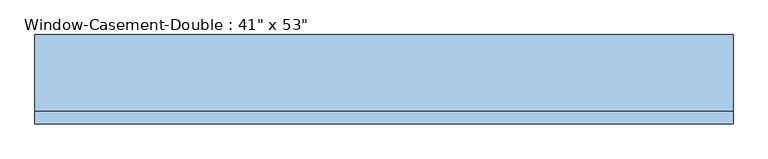
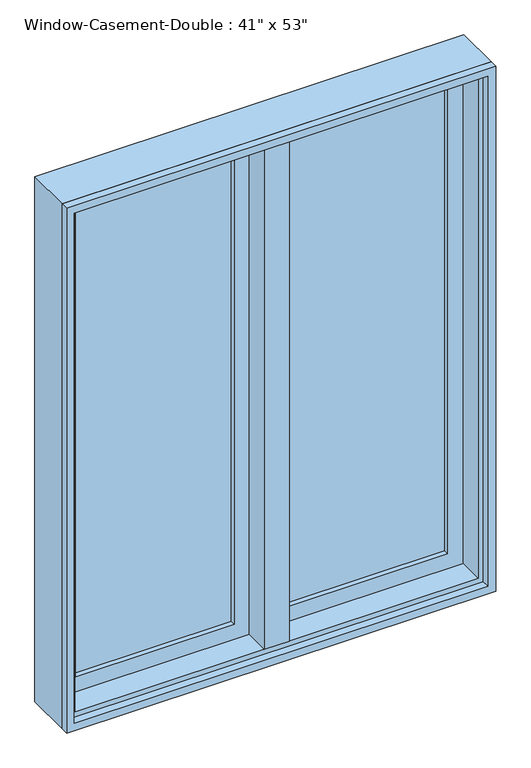
"""IFC4 building model written with IfcOpenShell, lengths in millimetres: window geometry."""

from ifc_helpers import new_model, si_unit, frame, origin, place, context, project, spatial, polyline, outline, extrude, faceted_brep, source, transform, mapped, element, save


def window_8ddb865a(model_context):
    return source(origin(), model_context, "Body", "SolidModel", [
        faceted_brep([(9.525, 76.2, 2247.9), (-9.525, 76.2, 2247.9), (-9.525, 25.4, 2247.9), (9.525, 25.4, 2247.9), (9.525, 76.2, 927.1), (9.525, 25.4, 927.1), (-9.525, 25.4, 927.1), (-9.525, 76.2, 927.1), (-9.525, 25.4, 946.15), (-9.525, 25.4, 2228.85), (-30.1625, 25.4, 946.15), (-30.1625, 25.4, 2228.85), (-30.1625, -38.1, 946.15), (-30.1625, -38.1, 2228.85), (30.1625, -38.1, 946.15), (30.1625, -38.1, 2228.85), (30.1625, 25.4, 946.15), (30.1625, 25.4, 2228.85), (9.525, 25.4, 946.15), (9.525, 25.4, 2228.85)], [[[0, 1, 2, 3]], [[4, 5, 6, 7]], [[1, 0, 4, 7]], [[2, 1, 7, 6, 8, 9]], [[9, 8, 10, 11]], [[11, 10, 12, 13]], [[13, 12, 14, 15]], [[15, 14, 16, 17]], [[17, 16, 18, 19]], [[0, 3, 19, 18, 5, 4]], [[18, 8, 6, 5]], [[9, 19, 3, 2]], [[8, 18, 16, 14, 12, 10]], [[19, 9, 11, 13, 15, 17]]]),
        extrude(outline(polyline([(-66.675, 57.15), (-66.675, 50.8), (-450.85, 50.8), (-450.85, 57.15), (-66.675, 57.15)])), frame((0.0, 0.0, 984.25), z_axis=(0.0, 0.0, 1.0), x_axis=(1.0, 0.0, 0.0)), (0.0, 0.0, 1.0), 1206.5),
        extrude(outline(polyline([(-450.85, 38.1), (-450.85, 44.45), (-66.675, 44.45), (-66.675, 38.1), (-450.85, 38.1)])), frame((0.0, 0.0, 984.25), z_axis=(0.0, 0.0, 1.0), x_axis=(1.0, 0.0, 0.0)), (0.0, 0.0, 1.0), 1206.5),
        extrude(outline(polyline([(450.85, 57.15), (450.85, 50.8), (66.675, 50.8), (66.675, 57.15), (450.85, 57.15)])), frame((0.0, 0.0, 984.25), z_axis=(0.0, 0.0, 1.0), x_axis=(1.0, 0.0, 0.0)), (0.0, 0.0, 1.0), 1206.5),
        extrude(outline(polyline([(66.675, 38.1), (66.675, 44.45), (450.85, 44.45), (450.85, 38.1), (66.675, 38.1)])), frame((0.0, 0.0, 984.25), z_axis=(0.0, 0.0, 1.0), x_axis=(1.0, 0.0, 0.0)), (0.0, 0.0, 1.0), 1206.5),
        extrude(outline(polyline([(2247.9, -508.0), (927.1, -508.0), (927.1, -9.525), (2247.9, -9.525), (2247.9, -508.0)]), holes=[polyline([(2190.75, -66.675), (984.25, -66.675), (984.25, -450.85), (2190.75, -450.85), (2190.75, -66.675)])]), frame((0.0, 25.4, 0.0), z_axis=(0.0, 1.0, 0.0), x_axis=(0.0, 0.0, 1.0)), (0.0, 0.0, 1.0), 44.45),
        extrude(outline(polyline([(927.1, 508.0), (2247.9, 508.0), (2247.9, 9.525), (927.1, 9.525), (927.1, 508.0)]), holes=[polyline([(984.25, 66.675), (2190.75, 66.675), (2190.75, 450.85), (984.25, 450.85), (984.25, 66.675)])]), frame((0.0, 25.4, 0.0), z_axis=(0.0, 1.0, 0.0), x_axis=(0.0, 0.0, 1.0)), (0.0, 0.0, 1.0), 44.45),
        extrude(outline(polyline([(2260.6, -520.7), (914.4, -520.7), (914.4, 520.7), (2260.6, 520.7), (2260.6, -520.7)]), holes=[polyline([(2241.55, 501.65), (933.45, 501.65), (933.45, -501.65), (2241.55, -501.65), (2241.55, 501.65)])]), frame((0.0, -57.15, 0.0), z_axis=(0.0, 1.0, 0.0), x_axis=(0.0, 0.0, 1.0)), (0.0, 0.0, 1.0), 19.05),
        faceted_brep([(488.95, 25.4, 2228.85), (488.95, -38.1, 2228.85), (-488.95, -38.1, 2228.85), (-488.95, 25.4, 2228.85), (508.0, 76.2, 2247.9), (508.0, 25.4, 2247.9), (-508.0, 25.4, 2247.9), (-508.0, 76.2, 2247.9), (520.7, -38.1, 2260.6), (520.7, 76.2, 2260.6), (-520.7, 76.2, 2260.6), (-520.7, -38.1, 2260.6), (-488.95, -38.1, 946.15), (-488.95, 25.4, 946.15), (-508.0, 25.4, 927.1), (-508.0, 76.2, 927.1), (-520.7, 76.2, 914.4), (-520.7, -38.1, 914.4), (488.95, -38.1, 946.15), (488.95, 25.4, 946.15), (508.0, 25.4, 927.1), (508.0, 76.2, 927.1), (520.7, 76.2, 914.4), (520.7, -38.1, 914.4)], [[[0, 1, 2, 3]], [[4, 5, 6, 7]], [[8, 9, 10, 11]], [[3, 2, 12, 13]], [[7, 6, 14, 15]], [[11, 10, 16, 17]], [[13, 12, 18, 19]], [[15, 14, 20, 21]], [[17, 16, 22, 23]], [[11, 17, 23, 8], [1, 18, 12, 2]], [[19, 18, 1, 0]], [[5, 20, 14, 6], [3, 13, 19, 0]], [[21, 20, 5, 4]], [[23, 22, 9, 8]], [[9, 22, 16, 10], [7, 15, 21, 4]]]),
    ])


if __name__ == "__main__":
    model = new_model("IFC4")
    model_context = context("Model", 3, world=origin())
    ifc_project = project(units=[si_unit("LENGTHUNIT", "METRE", prefix="MILLI")], contexts=[model_context])
    site = spatial("IfcSite", under=ifc_project)
    building = spatial("IfcBuilding", under=site)
    placement = place(None, origin())
    window_shape = window_8ddb865a(model_context)
    element("IfcWindow", 1, ObjectType="Window-Casement-Double : 41\" x 53\"", at=placement, inside=building, context=model_context, shape_type="MappedRepresentation", body=[
        mapped(window_shape, transform((0.0, 0.0, 0.0), x_axis=(1.0, 0.0, 0.0), y_axis=(0.0, 1.0, 0.0), z_axis=(0.0, 0.0, 1.0))),
    ])
    save(model, "model.ifc")

# Revit data of these elements
# Type "Window-Casement-Double : 41\" x 53\""
#   Type Mark = "15"
#   Fire Rating = "0.5h"
#   Assembly Code = "B2020100"
#   Analytic Construction = "Double glazing - domestic"
#   Frame Extension [instance default] = 0' - 0 1/4"
#   Window Inset [instance default] = 0' - 0"
#   Wall Thickness [instance default] = 0' - 6"
#   Interior Wall Closure [instance default] = 0' - 2 1/4"
#   Half Width = 1' - 8 1/2"
#   Visual Light Transmittance = 0.81
#   Thermal Resistance (R) = 1.8146 (h·ft²·°F)/BTU
#   Solar Heat Gain Coefficient = 0.76
#   Rough Width = 3' - 5 1/2"
#   Rough Height = 4' - 5 1/2"
#   Height = 4' - 5"
#   Heat Transfer Coefficient (U) = 0.5511 BTU/(h·ft²·°F)
#   Exterior Wall Closure [instance default] = 0' - 1 1/4"
#   Extension Jamb [instance default] = 0' - 2 1/4"
#   Default Sill Height = 3' - 0"
#   Width = 3' - 5"
#   Define Thermal Properties by = 0
#   Muntin Visibility = yes
#   Interior Trim Visibility [instance default] = yes
#   Exterior Trim Visibility [instance default] = yes
#   Extension Jamb Visibility [instance default] = yes
#   Interior Trim Material = Wood - Stained
#   Muntin Pattern = Muntin Pattern_2x2 : Muntin Pattern_2x2
#   Interior Trim = Trim-Window-Interior-Flat : Picture Frame
#   Interior Frame Material = Wood - Stained
#   Glass Panel Material = Glass
#   Exterior Trim Material = Clad - White
#   Exterior Trim = Trim-Window-Exterior-Flat : with Sill
#   Exterior Frame Material = Clad - White
#   Wall Closure = (empty or 0)
# Element 1 (IfcWindow, "Window-Casement-Double : 41\" x 53\"")
#   Wall Thickness = 0' - 4 1/2"
#   Extension Jamb = 0' - 0 3/4"
#   Materials on its faces: "Wood - Stained", "Glass", "Clad - White"
# Materials
#   "Wood - Stained": class "Wood", colour RGB 224 178 126, transparency 0, Cost = 0
#   "Glass": class "Glass", colour RGB 0 128 192, transparency 0.75, Description = "Soda Lime Glass", Cost = 0
#   "Clad - White": class "Wood", colour RGB 242 242 238, transparency 0, Cost = 0
